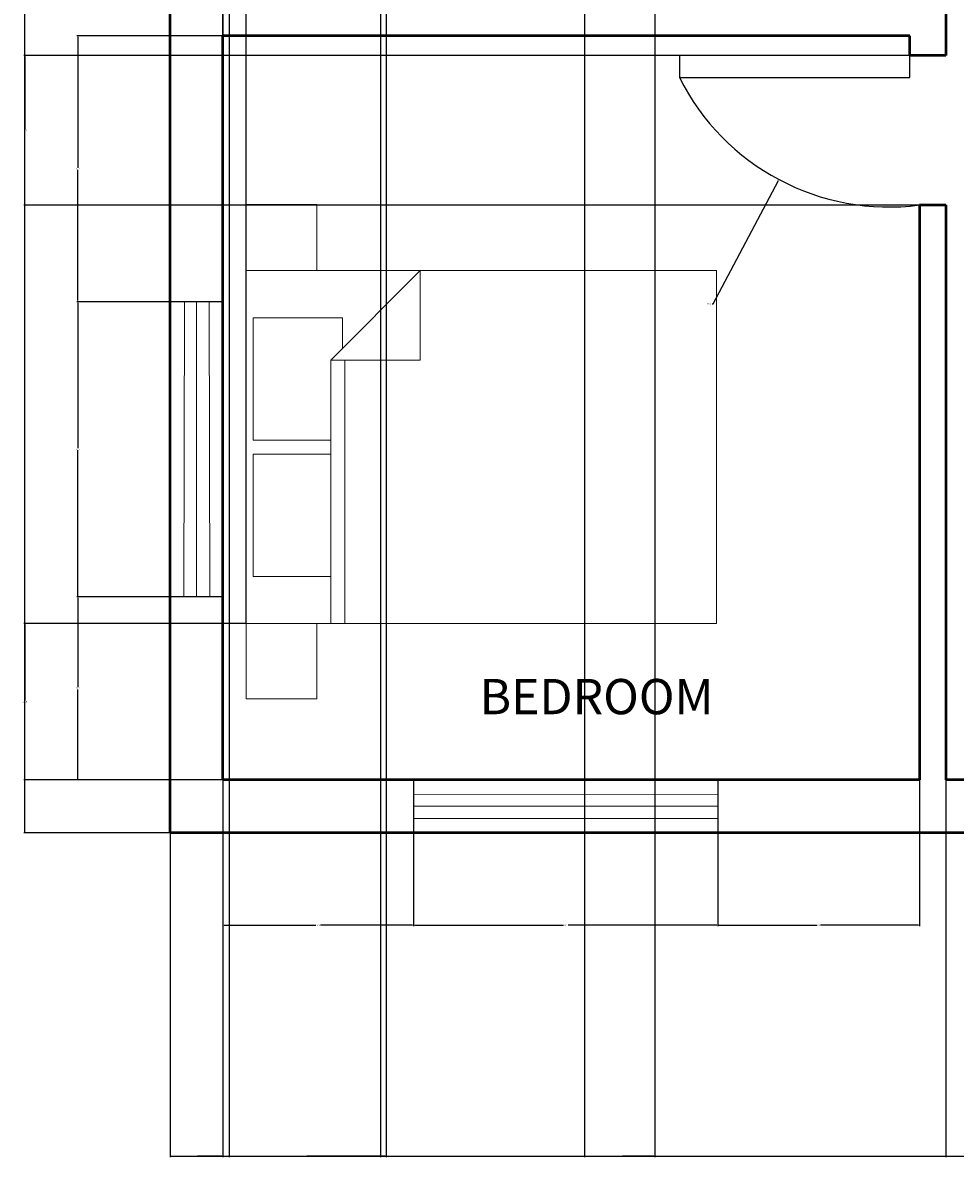
# Model space of a CAD drawing. Units: inches. Extents: x 1926 to 2293, y 1738 to 2280.
# Tile 1 of 6: x 1926 to 2084, y 1738 to 1931. Entities that reach past the tile are written whole.
import ezdxf

# ---------------------------------------------------------------- set-up
doc = ezdxf.new("R2010")
doc.units = ezdxf.units.IN
for name, color, linetype, lineweight in [('A-ANNO-DIMS', 2, 'Continuous', 18), ('A-AREA-IDEN', 7, 'Continuous', 25), ('A-DOOR', 3, 'Continuous', 25), ('A-FURN', 8, 'Continuous', 18), ('A-GLAZ', 4, 'Continuous', 18), ('A-WALL', 7, 'Continuous', 50)]:
    doc.layers.add(name, color=color, linetype=linetype, lineweight=lineweight)
doc.styles.get("Standard").update_dxf_attribs({"font": 'arial.ttf'})
doc.dimstyles.get("Standard").update_dxf_attribs({"dimtxt": 0.18, "dimasz": 0.18, "dimexe": 0.18, "dimexo": 0.0625, "dimgap": 0.09, "dimtad": 0, "dimtih": 1, "dimtoh": 1, "dimdec": 4, "dimzin": 0, "dimdsep": 46, "dimtxsty": 'Standard', "dimcen": 0.09, "dimadec": 0, "dimazin": 0, "dimtfac": 1, "dimtdec": 4, "dimtofl": 0, "dimtmove": 0, "dimatfit": 3, "dimfxl": 1, "dimtolj": 1, "dimtzin": 0, "dimarcsym": 0})

# ---------------------------------------------------------------- blocks, each defined once
blk = doc.blocks.new('Bed - Queen')
for p, q in [((0, -80.00003), (0, 0)), ((0, 0), (59.99999, 0)), ((59.99999, 0), (59.99999, -80.00003)), ((7.99999, -1.2), (28.79998, -1.2)), ((7.99999, -14.4), (7.99999, -1.2)), ((28.79998, -1.2), (28.79998, -14.4)), ((31.19999, -1.2), (51.99999, -1.2)), ((31.19999, -14.4), (31.19999, -1.2)), ((51.99999, -1.2), (51.99999, -16.4)), ((0, -14.4), (44.8, -14.4)), ((59.99999, -29.6), (44.8, -14.4)), ((44.8, -14.4), (44.8, -29.6)), ((44.8, -16.8), (0, -16.8)), ((51.99999, -16.4), (46.79936, -16.4)), ((44.8, -29.6), (59.99999, -29.6)), ((59.99999, -80.00003), (0, -80.00003))]:
    blk.add_line(p, q)
blk = doc.blocks.new('*D25')
at = {"layer": 'A-ANNO-DIMS', "color": 0, "lineweight": -2, "transparency": 16777216}
for p, q in [((1959.76, 1802.1), (1959.76, 1777.28)), ((1992.2, 1802.1), (1992.2, 1777.28)), ((1959.94, 1777.46), (1975.58, 1777.46)), ((1992.02, 1777.46), (1976.37, 1777.46))]:
    blk.add_line(p, q, dxfattribs=at)
at = {"layer": 'A-ANNO-DIMS', "color": 0, "transparency": 16777216}
for points in [[(1959.94, 1777.49), (1959.94, 1777.43), (1959.76, 1777.46)], [(1992.02, 1777.49), (1992.02, 1777.43), (1992.2, 1777.46)]]:
    blk.add_solid(points, dxfattribs=at)
at = {"layer": 'Defpoints', "color": 0, "transparency": 16777216}
for p in [(1959.76, 1802.16), (1992.2, 1802.16), (1959.76, 1777.46)]:
    blk.add_point(p, dxfattribs=at)
at = {"layer": 'A-ANNO-DIMS', "color": 0, "transparency": 16777216, "insert": (1975.98, 1777.46), "char_height": 0.18, "attachment_point": 5}
blk.add_mtext('\\A1;32.44', dxfattribs=at)
blk = doc.blocks.new('*D26')
at = {"layer": 'A-ANNO-DIMS', "color": 0, "lineweight": -2, "transparency": 16777216}
for p, q in [((1992.2, 1802.1), (1992.2, 1777.28)), ((2043.96, 1802.1), (2043.96, 1777.28)), ((1992.38, 1777.46), (2017.68, 1777.46)), ((2043.78, 1777.46), (2018.47, 1777.46))]:
    blk.add_line(p, q, dxfattribs=at)
at = {"layer": 'A-ANNO-DIMS', "color": 0, "transparency": 16777216}
for points in [[(1992.38, 1777.49), (1992.38, 1777.43), (1992.2, 1777.46)], [(2043.78, 1777.49), (2043.78, 1777.43), (2043.96, 1777.46)]]:
    blk.add_solid(points, dxfattribs=at)
at = {"layer": 'Defpoints', "color": 0, "transparency": 16777216}
for p in [(1992.2, 1802.16), (2043.96, 1802.16), (1992.2, 1777.46)]:
    blk.add_point(p, dxfattribs=at)
at = {"layer": 'A-ANNO-DIMS', "color": 0, "transparency": 16777216, "insert": (2018.08, 1777.46), "char_height": 0.18, "attachment_point": 5}
blk.add_mtext('\\A1;51.76', dxfattribs=at)
blk = doc.blocks.new('*D27')
at = {"layer": 'A-ANNO-DIMS', "color": 0, "lineweight": -2, "transparency": 16777216}
for p, q in [((2043.96, 1802.1), (2043.96, 1777.28)), ((2078.26, 1802.1), (2078.26, 1777.28)), ((2044.14, 1777.46), (2060.78, 1777.46)), ((2078.08, 1777.46), (2061.43, 1777.46))]:
    blk.add_line(p, q, dxfattribs=at)
at = {"layer": 'A-ANNO-DIMS', "color": 0, "transparency": 16777216}
for points in [[(2044.14, 1777.49), (2044.14, 1777.43), (2043.96, 1777.46)], [(2078.08, 1777.49), (2078.08, 1777.43), (2078.26, 1777.46)]]:
    blk.add_solid(points, dxfattribs=at)
at = {"layer": 'Defpoints', "color": 0, "transparency": 16777216}
for p in [(2043.96, 1802.16), (2078.26, 1802.16), (2043.96, 1777.46)]:
    blk.add_point(p, dxfattribs=at)
at = {"layer": 'A-ANNO-DIMS', "color": 0, "transparency": 16777216, "insert": (2061.11, 1777.46), "char_height": 0.18, "attachment_point": 5}
blk.add_mtext('\\A1;34.3', dxfattribs=at)
blk = doc.blocks.new('*D28')
at = {"layer": 'A-ANNO-DIMS', "color": 0, "lineweight": -2, "transparency": 16777216}
for p, q in [((2082.76, 1802.1), (2082.76, 1737.97)), ((2091.96, 1802.1), (2091.96, 1737.97)), ((2082.94, 1738.15), (2087.1, 1738.15)), ((2091.78, 1738.15), (2087.61, 1738.15))]:
    blk.add_line(p, q, dxfattribs=at)
at = {"layer": 'A-ANNO-DIMS', "color": 0, "transparency": 16777216}
for points in [[(2082.94, 1738.18), (2082.94, 1738.12), (2082.76, 1738.15)], [(2091.78, 1738.18), (2091.78, 1738.12), (2091.96, 1738.15)]]:
    blk.add_solid(points, dxfattribs=at)
at = {"layer": 'Defpoints', "color": 0, "transparency": 16777216}
for p in [(2082.76, 1802.16), (2091.96, 1802.16), (2091.96, 1738.15)]:
    blk.add_point(p, dxfattribs=at)
at = {"layer": 'A-ANNO-DIMS', "color": 0, "transparency": 16777216, "insert": (2087.36, 1738.15), "char_height": 0.18, "attachment_point": 5}
blk.add_mtext('\\A1;9.2', dxfattribs=at)
blk = doc.blocks.new('*D36')
at = {"layer": 'A-ANNO-DIMS', "color": 0, "lineweight": -2, "transparency": 16777216}
for p, q in [((1959.69, 1833.29), (1934.88, 1833.29)), ((1935.06, 1833.11), (1935.06, 1817.91)), ((1935.06, 1802.34), (1935.06, 1817.54)), ((1959.69, 1802.16), (1934.88, 1802.16))]:
    blk.add_line(p, q, dxfattribs=at)
at = {"layer": 'A-ANNO-DIMS', "color": 0, "transparency": 16777216}
for points in [[(1935.03, 1833.11), (1935.09, 1833.11), (1935.06, 1833.29)], [(1935.03, 1802.34), (1935.09, 1802.34), (1935.06, 1802.16)]]:
    blk.add_solid(points, dxfattribs=at)
at = {"layer": 'Defpoints', "color": 0, "transparency": 16777216}
for p in [(1935.06, 1833.29), (1959.76, 1833.29), (1959.76, 1802.16)]:
    blk.add_point(p, dxfattribs=at)
at = {"layer": 'A-ANNO-DIMS', "color": 0, "transparency": 16777216, "insert": (1935.06, 1817.73), "char_height": 0.18, "attachment_point": 5}
blk.add_mtext('\\A1;31.13', dxfattribs=at)
blk = doc.blocks.new('*D37')
at = {"layer": 'A-ANNO-DIMS', "color": 0, "lineweight": -2, "transparency": 16777216}
for p, q in [((1959.69, 1883.47), (1934.88, 1883.47)), ((1935.06, 1883.29), (1935.06, 1858.56)), ((1935.06, 1833.47), (1935.06, 1858.2)), ((1959.69, 1833.29), (1934.88, 1833.29))]:
    blk.add_line(p, q, dxfattribs=at)
at = {"layer": 'A-ANNO-DIMS', "color": 0, "transparency": 16777216}
for points in [[(1935.03, 1883.29), (1935.09, 1883.29), (1935.06, 1883.47)], [(1935.03, 1833.47), (1935.09, 1833.47), (1935.06, 1833.29)]]:
    blk.add_solid(points, dxfattribs=at)
at = {"layer": 'Defpoints', "color": 0, "transparency": 16777216}
for p in [(1935.06, 1883.47), (1959.76, 1883.47), (1959.76, 1833.29)]:
    blk.add_point(p, dxfattribs=at)
at = {"layer": 'A-ANNO-DIMS', "color": 0, "transparency": 16777216, "insert": (1935.06, 1858.38), "char_height": 0.18, "attachment_point": 5}
blk.add_mtext('\\A1;50.18', dxfattribs=at)
blk = doc.blocks.new('*D38')
at = {"layer": 'A-ANNO-DIMS', "color": 0, "lineweight": -2, "transparency": 16777216}
for p, q in [((1959.69, 1928.66), (1934.88, 1928.66)), ((1935.06, 1928.48), (1935.06, 1906.25)), ((1935.06, 1883.65), (1935.06, 1905.89)), ((1959.69, 1883.47), (1934.88, 1883.47))]:
    blk.add_line(p, q, dxfattribs=at)
at = {"layer": 'A-ANNO-DIMS', "color": 0, "transparency": 16777216}
for points in [[(1935.03, 1928.48), (1935.09, 1928.48), (1935.06, 1928.66)], [(1935.03, 1883.65), (1935.09, 1883.65), (1935.06, 1883.47)]]:
    blk.add_solid(points, dxfattribs=at)
at = {"layer": 'Defpoints', "color": 0, "transparency": 16777216}
for p in [(1935.06, 1928.66), (1959.76, 1928.66), (1959.76, 1883.47)]:
    blk.add_point(p, dxfattribs=at)
at = {"layer": 'A-ANNO-DIMS', "color": 0, "transparency": 16777216, "insert": (1935.06, 1906.07), "char_height": 0.18, "attachment_point": 5}
blk.add_mtext('\\A1;45.19', dxfattribs=at)
blk = doc.blocks.new('*D47')
at = {"layer": 'A-ANNO-DIMS', "color": 0, "lineweight": -2, "transparency": 16777216}
for p, q in [((1950.76, 2036.47), (1950.76, 1737.97)), ((1959.76, 2036.47), (1959.76, 1737.97)), ((1950.94, 1738.15), (1955.11, 1738.15)), ((1959.58, 1738.15), (1955.41, 1738.15))]:
    blk.add_line(p, q, dxfattribs=at)
at = {"layer": 'A-ANNO-DIMS', "color": 0, "transparency": 16777216}
for points in [[(1950.94, 1738.18), (1950.94, 1738.12), (1950.76, 1738.15)], [(1959.58, 1738.18), (1959.58, 1738.12), (1959.76, 1738.15)]]:
    blk.add_solid(points, dxfattribs=at)
at = {"layer": 'Defpoints', "color": 0, "transparency": 16777216}
for p in [(1950.76, 2036.53), (1959.76, 2036.53), (1959.76, 1738.15)]:
    blk.add_point(p, dxfattribs=at)
at = {"layer": 'A-ANNO-DIMS', "color": 0, "transparency": 16777216, "insert": (1955.26, 1738.15), "char_height": 0.18, "attachment_point": 5}
blk.add_mtext('\\A1;9', dxfattribs=at)
blk = doc.blocks.new('*D51')
at = {"layer": 'A-ANNO-DIMS', "color": 0, "lineweight": -2, "transparency": 16777216}
for p, q in [((1959.76, 2012.1), (1959.76, 1737.97)), ((1987.52, 2012.1), (1987.52, 1737.97)), ((1959.94, 1738.15), (1973.24, 1738.15)), ((1987.34, 1738.15), (1974.03, 1738.15))]:
    blk.add_line(p, q, dxfattribs=at)
at = {"layer": 'A-ANNO-DIMS', "color": 0, "transparency": 16777216}
for points in [[(1959.94, 1738.18), (1959.94, 1738.12), (1959.76, 1738.15)], [(1987.34, 1738.18), (1987.34, 1738.12), (1987.52, 1738.15)]]:
    blk.add_solid(points, dxfattribs=at)
at = {"layer": 'Defpoints', "color": 0, "transparency": 16777216}
for p in [(1959.76, 2012.16), (1987.52, 2012.16), (1987.52, 1738.15)]:
    blk.add_point(p, dxfattribs=at)
at = {"layer": 'A-ANNO-DIMS', "color": 0, "transparency": 16777216, "insert": (1973.64, 1738.15), "char_height": 0.18, "attachment_point": 5}
blk.add_mtext('\\A1;27.76', dxfattribs=at)
blk = doc.blocks.new('*D55')
at = {"layer": 'A-ANNO-DIMS', "color": 0, "lineweight": -2, "transparency": 16777216}
for p, q in [((1960.83, 2035.38), (1960.83, 1737.97)), ((1986.57, 2035.38), (1986.57, 1737.97)), ((1961.01, 1738.15), (1973.3, 1738.15)), ((1986.39, 1738.15), (1974.09, 1738.15))]:
    blk.add_line(p, q, dxfattribs=at)
at = {"layer": 'A-ANNO-DIMS', "color": 0, "transparency": 16777216}
for points in [[(1961.01, 1738.18), (1961.01, 1738.12), (1960.83, 1738.15)], [(1986.39, 1738.18), (1986.39, 1738.12), (1986.57, 1738.15)]]:
    blk.add_solid(points, dxfattribs=at)
at = {"layer": 'Defpoints', "color": 0, "transparency": 16777216}
for p in [(1960.83, 2035.45), (1986.57, 2035.45), (1986.57, 1738.15)]:
    blk.add_point(p, dxfattribs=at)
at = {"layer": 'A-ANNO-DIMS', "color": 0, "transparency": 16777216, "insert": (1973.7, 1738.15), "char_height": 0.18, "attachment_point": 5}
blk.add_mtext('\\A1;25.74', dxfattribs=at)
blk = doc.blocks.new('*D57')
at = {"layer": 'A-ANNO-DIMS', "color": 0, "lineweight": -2, "transparency": 16777216}
for p, q in [((2021.25, 2093.16), (2021.25, 1737.97)), ((2033.26, 2090.75), (2033.26, 1737.97)), ((2021.43, 1738.15), (2026.8, 1738.15)), ((2033.08, 1738.15), (2027.71, 1738.15))]:
    blk.add_line(p, q, dxfattribs=at)
at = {"layer": 'A-ANNO-DIMS', "color": 0, "transparency": 16777216}
for points in [[(2021.43, 1738.18), (2021.43, 1738.12), (2021.25, 1738.15)], [(2033.08, 1738.18), (2033.08, 1738.12), (2033.26, 1738.15)]]:
    blk.add_solid(points, dxfattribs=at)
at = {"layer": 'Defpoints', "color": 0, "transparency": 16777216}
for p in [(2021.25, 2093.23), (2033.26, 2090.81), (2033.26, 1738.15)]:
    blk.add_point(p, dxfattribs=at)
at = {"layer": 'A-ANNO-DIMS', "color": 0, "transparency": 16777216, "insert": (2027.26, 1738.15), "char_height": 0.18, "attachment_point": 5}
blk.add_mtext('\\A1;12.002', dxfattribs=at)
blk = doc.blocks.new('*D62')
at = {"layer": 'A-ANNO-DIMS', "color": 0, "lineweight": -2, "transparency": 16777216}
for p, q in [((2082.69, 1925.36), (1925.88, 1925.36)), ((1926.06, 1925.18), (1926.06, 1912.82)), ((1926.06, 1900.09), (1926.06, 1912.45)), ((2078.19, 1899.91), (1925.88, 1899.91))]:
    blk.add_line(p, q, dxfattribs=at)
at = {"layer": 'A-ANNO-DIMS', "color": 0, "transparency": 16777216}
for points in [[(1926.03, 1925.18), (1926.09, 1925.18), (1926.06, 1925.36)], [(1926.03, 1900.09), (1926.09, 1900.09), (1926.06, 1899.91)]]:
    blk.add_solid(points, dxfattribs=at)
at = {"layer": 'Defpoints', "color": 0, "transparency": 16777216}
for p in [(1926.06, 1925.36), (2082.76, 1925.36), (2078.26, 1899.91)]:
    blk.add_point(p, dxfattribs=at)
at = {"layer": 'A-ANNO-DIMS', "color": 0, "transparency": 16777216, "insert": (1926.06, 1912.63), "char_height": 0.18, "attachment_point": 5}
blk.add_mtext('\\A1;25.44', dxfattribs=at)
blk = doc.blocks.new('*D79')
at = {"layer": 'A-ANNO-DIMS', "color": 0, "lineweight": -2, "transparency": 16777216}
for p, q in [((1959.76, 1833.35), (1959.76, 2280.04)), ((1959.94, 2279.86), (1961.41, 2279.86)), ((1963.53, 2279.86), (1962.06, 2279.86)), ((1963.71, 1828.81), (1963.71, 2280.04))]:
    blk.add_line(p, q, dxfattribs=at)
at = {"layer": 'A-ANNO-DIMS', "color": 0, "transparency": 16777216}
for points in [[(1959.94, 2279.89), (1959.94, 2279.83), (1959.76, 2279.86)], [(1963.53, 2279.89), (1963.53, 2279.83), (1963.71, 2279.86)]]:
    blk.add_solid(points, dxfattribs=at)
at = {"layer": 'Defpoints', "color": 0, "transparency": 16777216}
for p in [(1959.76, 2279.86), (1959.76, 1833.29), (1963.71, 1828.75)]:
    blk.add_point(p, dxfattribs=at)
at = {"layer": 'A-ANNO-DIMS', "color": 0, "transparency": 16777216, "insert": (1961.74, 2279.86), "char_height": 0.18, "attachment_point": 5}
blk.add_mtext('\\A1;3.96', dxfattribs=at)
blk = doc.blocks.new('*D80')
at = {"layer": 'A-ANNO-DIMS', "color": 0, "lineweight": -2, "transparency": 16777216}
for p, q in [((1963.65, 1828.75), (1925.88, 1828.75)), ((1926.06, 1828.57), (1926.06, 1815.64)), ((1926.06, 1802.34), (1926.06, 1815.27)), ((1959.69, 1802.16), (1925.88, 1802.16))]:
    blk.add_line(p, q, dxfattribs=at)
at = {"layer": 'A-ANNO-DIMS', "color": 0, "transparency": 16777216}
for points in [[(1926.03, 1828.57), (1926.09, 1828.57), (1926.06, 1828.75)], [(1926.03, 1802.34), (1926.09, 1802.34), (1926.06, 1802.16)]]:
    blk.add_solid(points, dxfattribs=at)
at = {"layer": 'Defpoints', "color": 0, "transparency": 16777216}
for p in [(1963.71, 1828.75), (1926.06, 1802.16), (1959.76, 1802.16)]:
    blk.add_point(p, dxfattribs=at)
at = {"layer": 'A-ANNO-DIMS', "color": 0, "transparency": 16777216, "insert": (1926.06, 1815.45), "char_height": 0.18, "attachment_point": 5}
blk.add_mtext('\\A1;26.585', dxfattribs=at)
blk = doc.blocks.new('*D84')
at = {"layer": 'A-ANNO-DIMS', "color": 0, "lineweight": -2, "transparency": 16777216}
for p, q in [((1950.76, 1793.1), (1950.76, 1737.97)), ((2256.76, 1793.1), (2256.76, 1737.97)), ((1950.94, 1738.15), (2103.47, 1738.15)), ((2256.58, 1738.15), (2104.05, 1738.15))]:
    blk.add_line(p, q, dxfattribs=at)
at = {"layer": 'A-ANNO-DIMS', "color": 0, "transparency": 16777216}
for points in [[(1950.94, 1738.18), (1950.94, 1738.12), (1950.76, 1738.15)], [(2256.58, 1738.18), (2256.58, 1738.12), (2256.76, 1738.15)]]:
    blk.add_solid(points, dxfattribs=at)
at = {"layer": 'Defpoints', "color": 0, "transparency": 16777216}
for p in [(1950.76, 1793.16), (2256.76, 1793.16), (2256.76, 1738.15)]:
    blk.add_point(p, dxfattribs=at)
at = {"layer": 'A-ANNO-DIMS', "color": 0, "transparency": 16777216, "insert": (2103.76, 1738.15), "char_height": 0.18, "attachment_point": 5}
blk.add_mtext('\\A1;306', dxfattribs=at)
blk = doc.blocks.new('*D85')
at = {"layer": 'A-ANNO-DIMS', "color": 0, "lineweight": -2, "transparency": 16777216}
for p, q in [((1950.69, 2255.16), (1925.88, 2255.16)), ((1926.06, 2254.98), (1926.06, 2024.34)), ((1926.06, 1793.34), (1926.06, 2023.98)), ((1950.69, 1793.16), (1925.88, 1793.16))]:
    blk.add_line(p, q, dxfattribs=at)
at = {"layer": 'A-ANNO-DIMS', "color": 0, "transparency": 16777216}
for points in [[(1926.03, 2254.98), (1926.09, 2254.98), (1926.06, 2255.16)], [(1926.03, 1793.34), (1926.09, 1793.34), (1926.06, 1793.16)]]:
    blk.add_solid(points, dxfattribs=at)
at = {"layer": 'Defpoints', "color": 0, "transparency": 16777216}
for p in [(1926.06, 2255.16), (1950.76, 2255.16), (1950.76, 1793.16)]:
    blk.add_point(p, dxfattribs=at)
at = {"layer": 'A-ANNO-DIMS', "color": 0, "transparency": 16777216, "insert": (1926.06, 2024.16), "char_height": 0.18, "attachment_point": 5}
blk.add_mtext('\\A1;462', dxfattribs=at)
blk = doc.blocks.new('*D88')
at = {"layer": 'A-ANNO-DIMS', "color": 0, "lineweight": -2, "transparency": 16777216}
for p, q in [((2072.97, 1939.43), (2073.15, 1939.43)), ((2073.06, 1939.34), (2073.06, 1939.52)), ((2043.15, 1883.11), (2054.28, 1904.07)), ((2042.97, 1883.11), (2043.15, 1883.11))]:
    blk.add_line(p, q, dxfattribs=at)
at = {"layer": 'A-ANNO-DIMS', "color": 0, "transparency": 16777216}
blk.add_solid([(2054.26, 1904.08), (2054.31, 1904.06), (2054.37, 1904.23)], dxfattribs=at)
at = {"layer": 'Defpoints', "color": 0, "transparency": 16777216}
for p in [(2073.06, 1939.43), (2054.37, 1904.23)]:
    blk.add_point(p, dxfattribs=at)
at = {"layer": 'A-ANNO-DIMS', "color": 0, "transparency": 16777216, "insert": (2042.49, 1883.11), "char_height": 0.18, "attachment_point": 5}
blk.add_mtext('\\A1;R39.85', dxfattribs=at)

msp = doc.modelspace()

# ---------------------------------------------------------------- linework, layer by layer
at = {"layer": 'A-DOOR'}
for p, q in [((2076.6459, 1925.3552), (2037.4127, 1925.3552)), ((2037.4127, 1925.3552), (2037.4127, 1921.604)), ((2076.6459, 1921.604), (2076.6459, 1925.3552)), ((2037.4127, 1921.604), (2076.6459, 1921.604))]:
    msp.add_line(p, q, dxfattribs=at)
msp.add_arc((2073.0583, 1939.4257), 39.8525, 206.563628, 277.495312, dxfattribs=at)
at = {"layer": 'A-FURN'}
for points in [[(1963.7133, 1888.7469), (1975.7133, 1888.7469), (1975.7133, 1899.9722), (1963.7133, 1899.9722)], [(1963.7133, 1828.7469), (1975.7133, 1828.7469), (1975.7133, 1815.9516), (1963.7133, 1815.9516)]]:
    msp.add_lwpolyline(points, close=True, dxfattribs=at)
at = {"layer": 'A-GLAZ'}
for p, q in [((1953.1907, 1883.4728), (1953.0947, 1833.2892)), ((1955.2569, 1883.4728), (1955.2569, 1833.2892)), ((1957.4147, 1883.4728), (1957.5107, 1833.2892)), ((1992.1984, 1799.6863), (2043.9574, 1799.7466)), ((1992.1984, 1797.6622), (2043.9574, 1797.6622)), ((1992.1984, 1795.5849), (2043.9574, 1795.5849))]:
    msp.add_line(p, q, dxfattribs=at)
for points in [[(1950.7569, 1883.4728), (1959.7569, 1883.4728), (1959.7569, 1833.2892), (1950.7569, 1833.2892)], [(1992.1984, 1802.1622), (2043.9574, 1802.1622), (2043.9574, 1793.1622), (1992.1984, 1793.1622)]]:
    msp.add_lwpolyline(points, close=True, dxfattribs=at)
at = {"layer": 'A-WALL'}
for p, q in [((1950.7569, 1793.1622), (1950.7569, 2255.1622)), ((2082.7569, 1933.1622), (2082.7569, 1928.6622)), ((2082.7569, 1933.1622), (2082.7569, 1928.6622)), ((1959.7569, 1802.1622), (1959.7569, 1928.6622)), ((2076.6459, 1928.6622), (1959.7569, 1928.6622)), ((2076.6459, 1925.3552), (2076.6459, 1928.6622)), ((2082.7569, 1928.6622), (2082.7569, 1925.3552)), ((2082.7569, 1925.3552), (2076.6459, 1925.3552)), ((2078.2569, 1899.9137), (2082.7569, 1899.9137)), ((2078.2569, 1899.9137), (2078.2569, 1802.1622)), ((2082.7569, 1899.9137), (2082.7569, 1802.1622)), ((2082.7569, 1899.9137), (2082.7569, 1802.1622)), ((2078.2569, 1802.1622), (1959.7569, 1802.1622)), ((2091.9575, 1802.1622), (2082.7569, 1802.1622)), ((2091.9575, 1793.1622), (1950.7569, 1793.1622))]:
    msp.add_line(p, q, dxfattribs=at)

# ---------------------------------------------------------------- block references
at = {"layer": 'A-FURN', "rotation": 90}
msp.add_blockref('Bed - Queen', (1963.7133, 1828.7469), dxfattribs=at)

# ---------------------------------------------------------------- texts
at = {"layer": 'A-AREA-IDEN', "insert": (2003.412, 1819.3168), "char_height": 6, "attachment_point": 1}
msp.add_mtext_dynamic_manual_height_columns('BEDROOM', width=23.953264, gutter_width=12.5, heights=[0], dxfattribs=at)

# ---------------------------------------------------------------- dimensions: what is measured, and where the dimension line sits
at = {"layer": 'A-ANNO-DIMS'}
for base, p1, p2, override, picture, middle in [((1959.7569, 2279.8622), (1963.7133, 1828.7469), (1959.7569, 1833.2892), {"dimdec": 2, "dimlfac": 1, "dimrnd": 0, "dimzin": 0, "dimdsep": 46, "dimlunit": 2}, '*D79', (1961.7351, 2279.8622)), ((2033.2569, 1738.1524), (2021.2546, 2093.2275), (2033.2569, 2090.8146), {"dimdec": 3, "dimlfac": 1, "dimrnd": 0, "dimzin": 0, "dimdsep": 46, "dimlunit": 2}, '*D57', (2027.2557, 1738.1524)), ((1959.7569, 1738.1524), (1950.7569, 2036.5292), (1959.7569, 2036.5292), {"dimdec": 0, "dimlfac": 1, "dimrnd": 0, "dimzin": 0, "dimdsep": 46, "dimlunit": 2}, '*D47', (1955.2569, 1738.1524)), ((1986.5655, 1738.1524), (1960.8266, 2035.4453), (1986.5655, 2035.4453), {"dimdec": 2, "dimlfac": 1, "dimrnd": 0, "dimzin": 0, "dimdsep": 46, "dimlunit": 2}, '*D55', (1973.696, 1738.1524)), ((1987.5186, 1738.1524), (1959.7569, 2012.1622), (1987.5186, 2012.1622), {"dimdec": 2, "dimlfac": 1, "dimrnd": 0, "dimzin": 0, "dimdsep": 46, "dimlunit": 2}, '*D51', (1973.6378, 1738.1524)), ((2091.9575, 1738.1524), (2082.7569, 1802.1622), (2091.9575, 1802.1622), {"dimdec": 1, "dimlfac": 1, "dimrnd": 0, "dimzin": 0, "dimdsep": 46, "dimlunit": 2}, '*D28', (2087.3572, 1738.1524)), ((2256.7569, 1738.1524), (1950.7569, 1793.1622), (2256.7569, 1793.1622), {"dimdec": 0, "dimlfac": 1, "dimrnd": 0, "dimzin": 0, "dimdsep": 46, "dimlunit": 2}, '*D84', (2103.7569, 1738.1524))]:
    dim = msp.add_linear_dim(base=base, p1=p1, p2=p2, dimstyle='Standard', override=override, dxfattribs=at)
    dim.commit()
    dim.dimension.update_dxf_attribs({"geometry": picture, "text_midpoint": middle})
for base, p1, p2, angle, override, picture, middle in [((1926.0569, 2255.1622), (1950.7569, 1793.1622), (1950.7569, 2255.1622), 90, {"dimdec": 0, "dimlfac": 1, "dimrnd": 0, "dimzin": 0, "dimdsep": 46, "dimlunit": 2}, '*D85', (1926.0569, 2024.1622)), ((1935.0569, 1928.6622), (1959.7569, 1883.4728), (1959.7569, 1928.6622), 90, {"dimdec": 2, "dimlfac": 1, "dimrnd": 0, "dimzin": 0, "dimdsep": 46, "dimlunit": 2}, '*D38', (1935.0569, 1906.0675)), ((1926.0569, 1925.3552), (2078.2569, 1899.9137), (2082.7569, 1925.3552), 90, {"dimdec": 2, "dimlfac": 1, "dimrnd": 0, "dimzin": 0, "dimdsep": 46, "dimlunit": 2}, '*D62', (1926.0569, 1912.6345)), ((1935.0569, 1883.4728), (1959.7569, 1833.2892), (1959.7569, 1883.4728), 90, {"dimdec": 2, "dimlfac": 1, "dimrnd": 0, "dimzin": 0, "dimdsep": 46, "dimlunit": 2}, '*D37', (1935.0569, 1858.381)), ((1935.0569, 1833.2892), (1959.7569, 1802.1622), (1959.7569, 1833.2892), 90, {"dimdec": 2, "dimlfac": 1, "dimrnd": 0, "dimzin": 0, "dimdsep": 46, "dimlunit": 2}, '*D36', (1935.0569, 1817.7257)), ((1926.0569, 1802.1622), (1963.7133, 1828.7469), (1959.7569, 1802.1622), 90, {"dimdec": 3, "dimlfac": 1, "dimrnd": 0, "dimzin": 0, "dimdsep": 46, "dimlunit": 2}, '*D80', (1926.0569, 1815.4546)), ((1959.7569, 1777.4622), (1992.1984, 1802.1622), (1959.7569, 1802.1622), 180, {"dimdec": 2, "dimlfac": 1, "dimrnd": 0, "dimzin": 0, "dimdsep": 46, "dimlunit": 2}, '*D25', (1975.9776, 1777.4622)), ((1992.1984, 1777.4622), (2043.9574, 1802.1622), (1992.1984, 1802.1622), 180, {"dimdec": 2, "dimlfac": 1, "dimrnd": 0, "dimzin": 0, "dimdsep": 46, "dimlunit": 2}, '*D26', (2018.0779, 1777.4622)), ((2043.9574, 1777.4622), (2078.2569, 1802.1622), (2043.9574, 1802.1622), 180, {"dimdec": 1, "dimlfac": 1, "dimrnd": 0, "dimzin": 0, "dimdsep": 46, "dimlunit": 2}, '*D27', (2061.1071, 1777.4622))]:
    dim = msp.add_linear_dim(base=base, p1=p1, p2=p2, angle=angle, dimstyle='Standard', override=override, dxfattribs=at)
    dim.commit()
    dim.dimension.update_dxf_attribs({"geometry": picture, "text_midpoint": middle})
dim = msp.add_radius_dim(center=(2073.0583, 1939.4257), mpoint=(2054.3671, 1904.2282), dimstyle='Standard', override={"dimdec": 2, "dimlfac": 1, "dimrnd": 0, "dimzin": 0, "dimdsep": 46, "dimlunit": 2}, dxfattribs=at)
dim.commit()
dim.dimension.update_dxf_attribs({"geometry": '*D88', "text_midpoint": (2042.4919, 1883.1098), "dimtype": 164})

doc.saveas('drawing.dxf')
